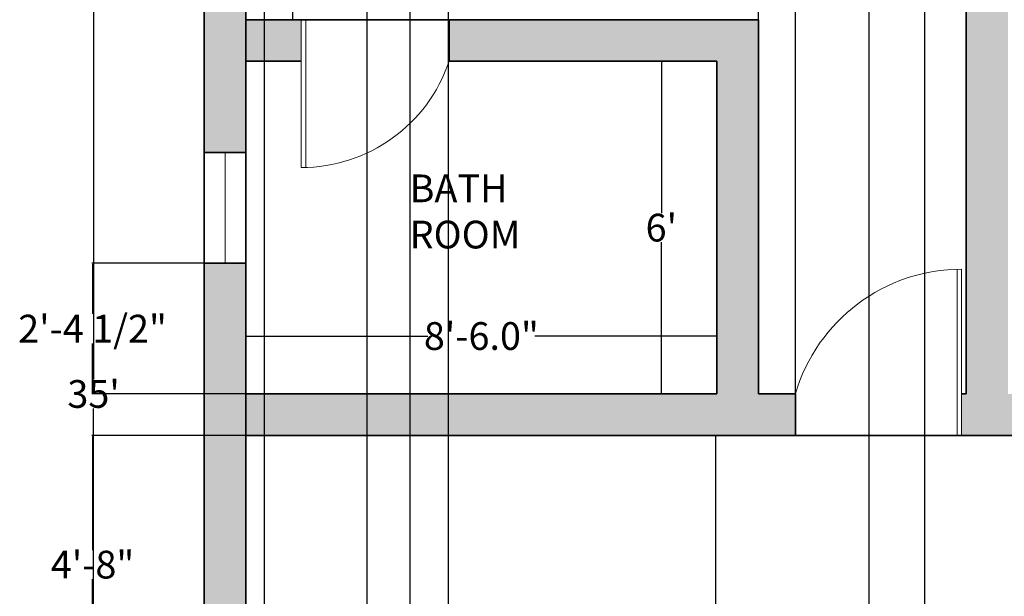
# Model space of a CAD drawing. Units: inches. Extents: x 1174 to 1615, y 3112 to 3628.
# Tile 3 of 6: x 1177 to 1390, y 3341 to 3466. Entities that reach past the tile are written whole.
import ezdxf

# ---------------------------------------------------------------- set-up
doc = ezdxf.new("R2010")
doc.units = ezdxf.units.IN
doc.header["$MEASUREMENT"] = 0
doc.layers.get('0').update_dxf_attribs({"color": 250})
for name, color, linetype, lineweight in [('A-ANNO-DIMS', 2, 'Continuous', 18), ('A-AREA-IDEN', 7, 'Continuous', 25), ('A-DOOR', 3, 'Continuous', 18), ('A-GLAZ', 4, 'Continuous', 18), ('A-WALL', 7, 'Continuous', 35)]:
    doc.layers.add(name, color=color, linetype=linetype, lineweight=lineweight)
doc.layers.add('A-WALL-PATT', color=18, linetype='Continuous', lineweight=13, true_color=0x000000)
doc.styles.get("Standard").update_dxf_attribs({"font": 'arial.ttf'})
doc.dimstyles.get("Standard").update_dxf_attribs({"dimtxt": 6, "dimasz": 0.18, "dimexe": 0.18, "dimexo": 0.0625, "dimgap": 0.09, "dimtad": 0, "dimtih": 1, "dimtoh": 1, "dimdec": 1, "dimzin": 0, "dimdsep": 46, "dimlunit": 3, "dimtxsty": 'Standard', "dimcen": 0.09, "dimadec": 0, "dimazin": 0, "dimtfac": 1, "dimtdec": 1, "dimtofl": 0, "dimtmove": 0, "dimatfit": 3, "dimfxl": 1, "dimtolj": 1, "dimtzin": 0, "dimarcsym": 0})

# ---------------------------------------------------------------- blocks, each defined once
blk = doc.blocks.new('*D4')
at = {"layer": 'A-ANNO-DIMS', "color": 0, "lineweight": -2, "transparency": 16777216}
for p, q in [((1216.6, 3595.03), (1192.51, 3595.03)), ((1192.69, 3594.85), (1192.69, 3388.18)), ((1192.69, 3175.21), (1192.69, 3381.87)), ((1216.6, 3175.03), (1192.51, 3175.03))]:
    blk.add_line(p, q, dxfattribs=at)
at = {"layer": 'A-ANNO-DIMS', "color": 0, "transparency": 16777216}
for points in [[(1192.66, 3594.85), (1192.72, 3594.85), (1192.69, 3595.03)], [(1192.66, 3175.21), (1192.72, 3175.21), (1192.69, 3175.03)]]:
    blk.add_solid(points, dxfattribs=at)
at = {"layer": 'Defpoints', "color": 0, "transparency": 16777216}
for p in [(1216.66, 3595.03), (1192.69, 3175.03), (1216.66, 3175.03)]:
    blk.add_point(p, dxfattribs=at)
at = {"layer": 'A-ANNO-DIMS', "color": 0, "transparency": 16777216, "insert": (1192.69, 3385.03), "char_height": 6, "attachment_point": 5}
blk.add_mtext("\\A1;35'", dxfattribs=at)
blk = doc.blocks.new('*D5')
at = {"layer": 'A-ANNO-DIMS', "color": 0, "lineweight": -2, "transparency": 16777216}
for p, q in [((1225.73, 3586.03), (1236.02, 3586.03)), ((1235.84, 3585.85), (1235.84, 3529.18)), ((1235.84, 3466.21), (1235.84, 3522.88)), ((1225.73, 3466.03), (1236.02, 3466.03))]:
    blk.add_line(p, q, dxfattribs=at)
at = {"layer": 'A-ANNO-DIMS', "color": 0, "transparency": 16777216}
for points in [[(1235.81, 3585.85), (1235.87, 3585.85), (1235.84, 3586.03)], [(1235.81, 3466.21), (1235.87, 3466.21), (1235.84, 3466.03)]]:
    blk.add_solid(points, dxfattribs=at)
at = {"layer": 'Defpoints', "color": 0, "transparency": 16777216}
for p in [(1225.66, 3586.03), (1225.66, 3466.03), (1235.84, 3466.03)]:
    blk.add_point(p, dxfattribs=at)
at = {"layer": 'A-ANNO-DIMS', "color": 0, "transparency": 16777216, "insert": (1235.84, 3526.03), "char_height": 6, "attachment_point": 5}
blk.add_mtext("\\A1;10'", dxfattribs=at)
blk = doc.blocks.new('*D7')
at = {"layer": 'A-ANNO-DIMS', "color": 0, "lineweight": -2, "transparency": 16777216}
for p, q in [((1225.66, 3385.09), (1225.66, 3397.75)), ((1225.84, 3397.57), (1265.1, 3397.57)), ((1327.48, 3397.57), (1288.23, 3397.57)), ((1327.66, 3385.09), (1327.66, 3397.75))]:
    blk.add_line(p, q, dxfattribs=at)
at = {"layer": 'A-ANNO-DIMS', "color": 0, "transparency": 16777216}
for points in [[(1225.84, 3397.6), (1225.84, 3397.54), (1225.66, 3397.57)], [(1327.48, 3397.6), (1327.48, 3397.54), (1327.66, 3397.57)]]:
    blk.add_solid(points, dxfattribs=at)
at = {"layer": 'Defpoints', "color": 0, "transparency": 16777216}
for p in [(1327.66, 3397.57), (1225.66, 3385.03), (1327.66, 3385.03)]:
    blk.add_point(p, dxfattribs=at)
at = {"layer": 'A-ANNO-DIMS', "color": 0, "transparency": 16777216, "insert": (1276.66, 3397.57), "char_height": 6, "attachment_point": 5}
blk.add_mtext('\\A1;8\'-6.0"', dxfattribs=at)
blk = doc.blocks.new('*D8')
at = {"layer": 'A-ANNO-DIMS', "color": 0, "lineweight": -2, "transparency": 16777216}
for p, q in [((1327.6, 3457.03), (1315.45, 3457.03)), ((1315.63, 3456.85), (1315.63, 3424.18)), ((1315.63, 3385.21), (1315.63, 3417.88)), ((1327.6, 3385.03), (1315.45, 3385.03))]:
    blk.add_line(p, q, dxfattribs=at)
at = {"layer": 'A-ANNO-DIMS', "color": 0, "transparency": 16777216}
for points in [[(1315.6, 3456.85), (1315.66, 3456.85), (1315.63, 3457.03)], [(1315.6, 3385.21), (1315.66, 3385.21), (1315.63, 3385.03)]]:
    blk.add_solid(points, dxfattribs=at)
at = {"layer": 'Defpoints', "color": 0, "transparency": 16777216}
for p in [(1327.66, 3457.03), (1315.63, 3385.03), (1327.66, 3385.03)]:
    blk.add_point(p, dxfattribs=at)
at = {"layer": 'A-ANNO-DIMS', "color": 0, "transparency": 16777216, "insert": (1315.63, 3421.03), "char_height": 6, "attachment_point": 5}
blk.add_mtext("\\A1;6'", dxfattribs=at)
blk = doc.blocks.new('*D18')
at = {"layer": 'A-ANNO-DIMS', "color": 0, "lineweight": -2, "transparency": 16777216}
for p, q in [((1225.73, 3376.03), (1327.55, 3376.03)), ((1327.37, 3375.85), (1327.37, 3283.18)), ((1327.37, 3184.21), (1327.37, 3276.88)), ((1225.73, 3184.03), (1327.55, 3184.03))]:
    blk.add_line(p, q, dxfattribs=at)
at = {"layer": 'A-ANNO-DIMS', "color": 0, "transparency": 16777216}
for points in [[(1327.34, 3375.85), (1327.4, 3375.85), (1327.37, 3376.03)], [(1327.34, 3184.21), (1327.4, 3184.21), (1327.37, 3184.03)]]:
    blk.add_solid(points, dxfattribs=at)
at = {"layer": 'Defpoints', "color": 0, "transparency": 16777216}
for p in [(1225.66, 3376.03), (1225.66, 3184.03), (1327.37, 3184.03)]:
    blk.add_point(p, dxfattribs=at)
at = {"layer": 'A-ANNO-DIMS', "color": 0, "transparency": 16777216, "insert": (1327.37, 3280.03), "char_height": 6, "attachment_point": 5}
blk.add_mtext("\\A1;16'", dxfattribs=at)
blk = doc.blocks.new('DOOR-SWING-36IN')
for p, q in [((-1, 36), (-1, 0)), ((0, 0), (0, 36)), ((0, 0), (-36, 0))]:
    blk.add_line(p, q)
blk.add_arc((0, -1.5), 37.5, 90, 163.7398)
blk = doc.blocks.new('DOOR-SWING-32IN')
for p, q in [((0, 0), (0, -32)), ((0, 0), (32, 0)), ((1, -32), (1, 0))]:
    blk.add_line(p, q)
blk.add_arc((0, 1.76), 33.76, 270, 341.4134)
blk = doc.blocks.new('VENT-WINDOW-24IN')
for p, q in [((-4.5, -24), (-4.5, 0)), ((0, 0), (0, -24)), ((4.5, 0), (4.5, -24))]:
    blk.add_line(p, q)
blk = doc.blocks.new('*D48')
at = {"layer": 'A-ANNO-DIMS', "color": 0, "lineweight": -2, "transparency": 16777216}
for p, q in [((1225.6, 3413.31), (1192.28, 3413.31)), ((1192.46, 3413.13), (1192.46, 3402.36)), ((1192.46, 3385.21), (1192.46, 3395.98)), ((1225.6, 3385.03), (1192.28, 3385.03))]:
    blk.add_line(p, q, dxfattribs=at)
at = {"layer": 'A-ANNO-DIMS', "color": 0, "transparency": 16777216}
for points in [[(1192.43, 3413.13), (1192.49, 3413.13), (1192.46, 3413.31)], [(1192.43, 3385.21), (1192.49, 3385.21), (1192.46, 3385.03)]]:
    blk.add_solid(points, dxfattribs=at)
at = {"layer": 'Defpoints', "color": 0, "transparency": 16777216}
for p in [(1192.46, 3413.31), (1225.66, 3413.31), (1225.66, 3385.03)]:
    blk.add_point(p, dxfattribs=at)
at = {"layer": 'A-ANNO-DIMS', "color": 0, "transparency": 16777216, "insert": (1192.46, 3399.17), "char_height": 6, "attachment_point": 5}
blk.add_mtext('\\A1;2\'-4 1/2"', dxfattribs=at)
blk = doc.blocks.new('*D49')
at = {"layer": 'A-ANNO-DIMS', "color": 0, "lineweight": -2, "transparency": 16777216}
for p, q in [((1225.73, 3376.03), (1589.04, 3376.03)), ((1588.86, 3375.85), (1588.86, 3351.02)), ((1588.86, 3319.81), (1588.86, 3344.64)), ((1225.73, 3319.63), (1589.04, 3319.63))]:
    blk.add_line(p, q, dxfattribs=at)
at = {"layer": 'A-ANNO-DIMS', "color": 0, "transparency": 16777216}
for points in [[(1588.83, 3375.85), (1588.89, 3375.85), (1588.86, 3376.03)], [(1588.83, 3319.81), (1588.89, 3319.81), (1588.86, 3319.63)]]:
    blk.add_solid(points, dxfattribs=at)
at = {"layer": 'Defpoints', "color": 0, "transparency": 16777216}
for p in [(1225.66, 3376.03), (1225.66, 3319.63), (1588.86, 3319.63)]:
    blk.add_point(p, dxfattribs=at)
at = {"layer": 'A-ANNO-DIMS', "color": 0, "transparency": 16777216, "insert": (1588.86, 3347.83), "char_height": 6, "attachment_point": 5}
blk.add_mtext('\\A1;4\'-8 1/2"', dxfattribs=at)
blk = doc.blocks.new('*D52')
at = {"layer": 'A-ANNO-DIMS', "color": 0, "lineweight": -2, "transparency": 16777216}
for p, q in [((1555.6, 3376.03), (1192.28, 3376.03)), ((1192.46, 3375.85), (1192.46, 3351.26)), ((1192.46, 3320.35), (1192.46, 3344.95)), ((1555.6, 3320.17), (1192.28, 3320.17))]:
    blk.add_line(p, q, dxfattribs=at)
at = {"layer": 'A-ANNO-DIMS', "color": 0, "transparency": 16777216}
for points in [[(1192.43, 3375.85), (1192.49, 3375.85), (1192.46, 3376.03)], [(1192.43, 3320.35), (1192.49, 3320.35), (1192.46, 3320.17)]]:
    blk.add_solid(points, dxfattribs=at)
at = {"layer": 'Defpoints', "color": 0, "transparency": 16777216}
for p in [(1555.66, 3376.03), (1192.46, 3320.17), (1555.66, 3320.17)]:
    blk.add_point(p, dxfattribs=at)
at = {"layer": 'A-ANNO-DIMS', "color": 0, "transparency": 16777216, "insert": (1192.46, 3348.1), "char_height": 6, "attachment_point": 5}
blk.add_mtext('\\A1;4\'-8"', dxfattribs=at)
blk = doc.blocks.new('*D56')
at = {"layer": 'A-ANNO-DIMS', "color": 0, "lineweight": -2, "transparency": 16777216}
for p, q in [((1336.66, 3385.09), (1336.66, 3619.41)), ((1336.84, 3619.23), (1344.48, 3619.23)), ((1344.66, 3385.09), (1344.66, 3619.41)), ((1344.66, 3619.23), (1344.84, 3619.23))]:
    blk.add_line(p, q, dxfattribs=at)
at = {"layer": 'A-ANNO-DIMS', "color": 0, "transparency": 16777216}
for points in [[(1336.84, 3619.26), (1336.84, 3619.2), (1336.66, 3619.23)], [(1344.48, 3619.26), (1344.48, 3619.2), (1344.66, 3619.23)]]:
    blk.add_solid(points, dxfattribs=at)
at = {"layer": 'Defpoints', "color": 0, "transparency": 16777216}
for p in [(1344.66, 3619.23), (1336.66, 3385.03), (1344.66, 3385.03)]:
    blk.add_point(p, dxfattribs=at)
at = {"layer": 'A-ANNO-DIMS', "color": 0, "transparency": 16777216, "insert": (1352.91, 3619.23), "char_height": 6, "attachment_point": 5}
blk.add_mtext('\\A1;0\'-8"', dxfattribs=at)
blk = doc.blocks.new('*D58')
at = {"layer": 'A-ANNO-DIMS', "color": 0, "lineweight": -2, "transparency": 16777216}
for p, q in [((1360.66, 3184.09), (1360.66, 3619.41)), ((1360.84, 3619.23), (1372.48, 3619.23)), ((1372.66, 3184.09), (1372.66, 3619.41)), ((1372.66, 3619.23), (1372.84, 3619.23))]:
    blk.add_line(p, q, dxfattribs=at)
at = {"layer": 'A-ANNO-DIMS', "color": 0, "transparency": 16777216}
for points in [[(1360.84, 3619.26), (1360.84, 3619.2), (1360.66, 3619.23)], [(1372.48, 3619.26), (1372.48, 3619.2), (1372.66, 3619.23)]]:
    blk.add_solid(points, dxfattribs=at)
at = {"layer": 'Defpoints', "color": 0, "transparency": 16777216}
for p in [(1372.66, 3619.23), (1360.66, 3184.03), (1372.66, 3184.03)]:
    blk.add_point(p, dxfattribs=at)
at = {"layer": 'A-ANNO-DIMS', "color": 0, "transparency": 16777216, "insert": (1380.63, 3619.23), "char_height": 6, "attachment_point": 5}
blk.add_mtext('\\A1;1\'-0"', dxfattribs=at)
blk = doc.blocks.new('*D60')
at = {"layer": 'A-ANNO-DIMS', "color": 0, "lineweight": -2, "transparency": 16777216}
for p, q in [((1229.72, 3290.15), (1229.72, 3619.41)), ((1229.9, 3619.23), (1230.72, 3619.23)), ((1251.77, 3619.23), (1250.95, 3619.23)), ((1251.95, 3292.11), (1251.95, 3619.41))]:
    blk.add_line(p, q, dxfattribs=at)
at = {"layer": 'A-ANNO-DIMS', "color": 0, "transparency": 16777216}
for points in [[(1229.9, 3619.26), (1229.9, 3619.2), (1229.72, 3619.23)], [(1251.77, 3619.26), (1251.77, 3619.2), (1251.95, 3619.23)]]:
    blk.add_solid(points, dxfattribs=at)
at = {"layer": 'Defpoints', "color": 0, "transparency": 16777216}
for p in [(1251.95, 3619.23), (1251.95, 3292.05), (1229.72, 3290.09)]:
    blk.add_point(p, dxfattribs=at)
at = {"layer": 'A-ANNO-DIMS', "color": 0, "transparency": 16777216, "insert": (1240.84, 3619.23), "char_height": 6, "attachment_point": 5}
blk.add_mtext('\\A1;1\'-10"', dxfattribs=at)
blk = doc.blocks.new('*D64')
at = {"layer": 'A-ANNO-DIMS', "color": 0, "lineweight": -2, "transparency": 16777216}
for p, q in [((1251.95, 3292.11), (1251.95, 3619.41)), ((1252.13, 3619.23), (1269.39, 3619.23)), ((1269.57, 3281.81), (1269.57, 3619.41)), ((1269.57, 3619.23), (1269.75, 3619.23))]:
    blk.add_line(p, q, dxfattribs=at)
at = {"layer": 'A-ANNO-DIMS', "color": 0, "transparency": 16777216}
for points in [[(1252.13, 3619.26), (1252.13, 3619.2), (1251.95, 3619.23)], [(1269.39, 3619.26), (1269.39, 3619.2), (1269.57, 3619.23)]]:
    blk.add_solid(points, dxfattribs=at)
at = {"layer": 'Defpoints', "color": 0, "transparency": 16777216}
for p in [(1269.57, 3619.23), (1251.95, 3292.05), (1269.57, 3281.75)]:
    blk.add_point(p, dxfattribs=at)
at = {"layer": 'A-ANNO-DIMS', "color": 0, "transparency": 16777216, "insert": (1284.52, 3619.23), "char_height": 6, "attachment_point": 5}
blk.add_mtext('\\A1;1\'-5 1/2"', dxfattribs=at)
blk = doc.blocks.new('*D69')
at = {"layer": 'A-ANNO-DIMS', "color": 0, "lineweight": -2, "transparency": 16777216}
for p, q in [((1225.66, 3585.97), (1225.66, 3120.65)), ((1261.16, 3585.86), (1261.16, 3120.65)), ((1225.84, 3120.83), (1225.98, 3120.83)), ((1260.98, 3120.83), (1260.85, 3120.83))]:
    blk.add_line(p, q, dxfattribs=at)
at = {"layer": 'A-ANNO-DIMS', "color": 0, "transparency": 16777216}
for points in [[(1225.84, 3120.86), (1225.84, 3120.8), (1225.66, 3120.83)], [(1260.98, 3120.86), (1260.98, 3120.8), (1261.16, 3120.83)]]:
    blk.add_solid(points, dxfattribs=at)
at = {"layer": 'Defpoints', "color": 0, "transparency": 16777216}
for p in [(1225.66, 3586.03), (1261.16, 3585.93), (1261.16, 3120.83)]:
    blk.add_point(p, dxfattribs=at)
at = {"layer": 'A-ANNO-DIMS', "color": 0, "transparency": 16777216, "insert": (1243.41, 3120.83), "char_height": 6, "attachment_point": 5}
blk.add_mtext('\\A1;2\'-11 1/2"', dxfattribs=at)
blk = doc.blocks.new('*D71')
at = {"layer": 'A-ANNO-DIMS', "color": 0, "lineweight": -2, "transparency": 16777216}
for p, q in [((1225.66, 3283.7), (1225.66, 3619.41)), ((1225.84, 3619.23), (1229.54, 3619.23)), ((1229.72, 3290.15), (1229.72, 3619.41)), ((1229.72, 3619.23), (1229.9, 3619.23))]:
    blk.add_line(p, q, dxfattribs=at)
at = {"layer": 'A-ANNO-DIMS', "color": 0, "transparency": 16777216}
for points in [[(1225.84, 3619.26), (1225.84, 3619.2), (1225.66, 3619.23)], [(1229.54, 3619.26), (1229.54, 3619.2), (1229.72, 3619.23)]]:
    blk.add_solid(points, dxfattribs=at)
at = {"layer": 'Defpoints', "color": 0, "transparency": 16777216}
for p in [(1229.72, 3619.23), (1229.72, 3290.09), (1225.66, 3283.63)]:
    blk.add_point(p, dxfattribs=at)
at = {"layer": 'A-ANNO-DIMS', "color": 0, "transparency": 16777216, "insert": (1237.97, 3619.23), "char_height": 6, "attachment_point": 5}
blk.add_mtext('\\A1;0\'-4"', dxfattribs=at)

msp = doc.modelspace()

# ---------------------------------------------------------------- hatches: boundary and pattern name
at = {"layer": 'A-WALL-PATT'}
h = msp.add_hatch(color=256, dxfattribs=at)
h.dxf.hatch_style = 1
h.paths.add_polyline_path([(1564.66, 3595.03), (1216.66, 3595.03), (1216.66, 3564.55), (1225.66, 3564.55), (1225.66, 3586.03), (1381.66, 3586.03), (1381.66, 3385.03), (1380.66, 3385.03), (1380.66, 3376.03), (1381.66, 3376.03), (1407.66, 3376.03), (1407.66, 3385.03), (1390.66, 3385.03), (1390.66, 3586.03), (1555.66, 3586.03), (1555.66, 3558.83), (1564.66, 3558.83)])
h.paths.add_polyline_path([(1564.66, 3408.64), (1555.66, 3408.64), (1555.66, 3385.03), (1453.66, 3385.03), (1453.66, 3457.03), (1465.66, 3457.03), (1465.66, 3466.03), (1453.66, 3466.03), (1444.66, 3466.03), (1444.66, 3385.03), (1443.66, 3385.03), (1443.66, 3376.03), (1444.66, 3376.03), (1555.66, 3376.03), (1555.66, 3320.17), (1564.66, 3320.17)])
h.paths.add_polyline_path([(1564.66, 3522.83), (1555.66, 3522.83), (1555.66, 3466.03), (1497.66, 3466.03), (1497.66, 3457.03), (1555.66, 3457.03), (1555.66, 3432.64), (1564.66, 3432.64)], flags=17)
h.paths.add_polyline_path([(1344.66, 3385.03), (1336.66, 3385.03), (1336.66, 3466.03), (1269.66, 3466.03), (1269.66, 3457.03), (1327.66, 3457.03), (1327.66, 3385.03), (1225.66, 3385.03), (1225.66, 3413.31), (1216.66, 3413.31), (1216.66, 3319.63), (1225.66, 3319.63), (1225.66, 3376.03), (1344.66, 3376.03)])
h.paths.add_polyline_path([(1237.66, 3466.03), (1225.66, 3466.03), (1225.66, 3528.55), (1216.66, 3528.55), (1216.66, 3437.31), (1225.66, 3437.31), (1225.66, 3457.03), (1237.66, 3457.03)], flags=17)
h.paths.add_polyline_path([(1265.25, 3184.03), (1225.66, 3184.03), (1225.66, 3283.63), (1216.66, 3283.63), (1216.66, 3175.03), (1265.25, 3175.03)])
h.paths.add_polyline_path([(1372.66, 3184.03), (1360.66, 3184.03), (1360.66, 3268.03), (1376.66, 3268.03), (1376.66, 3277.03), (1360.66, 3277.03), (1360.66, 3313.03), (1351.66, 3313.03), (1351.66, 3184.03), (1301.25, 3184.03), (1301.25, 3175.03), (1372.66, 3175.03)])
h.paths.add_polyline_path([(1460.02, 3184.03), (1429.66, 3184.03), (1429.66, 3277.03), (1408.66, 3277.03), (1408.66, 3268.03), (1420.66, 3268.03), (1420.66, 3184.03), (1408.66, 3184.03), (1408.66, 3175.03), (1460.02, 3175.03)])
h.paths.add_polyline_path([(1564.66, 3284.17), (1555.66, 3284.17), (1555.66, 3184.03), (1520.02, 3184.03), (1520.02, 3175.03), (1564.66, 3175.03)])

# ---------------------------------------------------------------- linework, layer by layer
at = {"layer": 'A-DOOR'}
for p, q in [((1237.66, 3434.03), (1237.66, 3466.03)), ((1380.66, 3412.03), (1380.66, 3376.03))]:
    msp.add_line(p, q, dxfattribs=at)
at = {"layer": 'A-WALL'}
for p, q in [((1216.66, 3595.03), (1216.66, 3175.03)), ((1225.66, 3586.03), (1225.66, 3466.03)), ((1381.66, 3586.03), (1381.66, 3385.03)), ((1225.66, 3466.03), (1336.66, 3466.03)), ((1225.66, 3466.03), (1237.66, 3466.03)), ((1269.66, 3466.03), (1269.66, 3457.03)), ((1336.66, 3466.03), (1336.66, 3385.03)), ((1225.66, 3457.03), (1237.66, 3457.03)), ((1225.66, 3457.03), (1225.66, 3385.03)), ((1269.66, 3457.03), (1327.66, 3457.03)), ((1327.66, 3457.03), (1327.66, 3385.03)), ((1216.66, 3437.31), (1225.66, 3437.31)), ((1225.66, 3413.31), (1216.66, 3413.31)), ((1225.66, 3385.03), (1327.66, 3385.03)), ((1336.66, 3385.03), (1344.66, 3385.03)), ((1344.66, 3376.03), (1344.66, 3385.03)), ((1380.66, 3385.03), (1381.66, 3385.03)), ((1225.66, 3376.03), (1555.66, 3376.03)), ((1225.66, 3376.03), (1225.66, 3184.03)), ((1381.66, 3376.03), (1380.66, 3376.03))]:
    msp.add_line(p, q, dxfattribs=at)

# ---------------------------------------------------------------- block references
at = {"layer": 'A-DOOR'}
for name, p in [('DOOR-SWING-32IN', (1237.66, 3466.03)), ('DOOR-SWING-36IN', (1380.66, 3376.03))]:
    msp.add_blockref(name, p, dxfattribs=at)
at = {"layer": 'A-GLAZ'}
msp.add_blockref('VENT-WINDOW-24IN', (1221.16, 3437.31), dxfattribs=at)

# ---------------------------------------------------------------- texts
at = {"layer": 'A-AREA-IDEN', "insert": (1261.12, 3432.53), "char_height": 6, "attachment_point": 1}
msp.add_mtext_dynamic_manual_height_columns('BATH \\PROOM', width=55.5508, gutter_width=1, heights=[0], dxfattribs=at)

# ---------------------------------------------------------------- dimensions: what is measured, and where the dimension line sits
at = {"layer": 'A-ANNO-DIMS'}
for base, p1, p2, override, picture, middle in [((1269.57, 3619.23), (1251.95, 3292.05), (1269.57, 3281.75), {"dimdec": 1, "dimlfac": 1, "dimrnd": 0, "dimzin": 1, "dimdsep": 46, "dimlunit": 4, "dimfrac": 2}, '*D64', (1284.52, 3619.23)), ((1229.72, 3619.23), (1225.66, 3283.63), (1229.72, 3290.09), {"dimdec": 1, "dimlfac": 1, "dimrnd": 0, "dimzin": 1, "dimdsep": 46, "dimlunit": 4, "dimfrac": 2}, '*D71', (1237.97, 3619.23)), ((1251.95, 3619.23), (1229.72, 3290.09), (1251.95, 3292.05), {"dimdec": 1, "dimlfac": 1, "dimrnd": 0, "dimzin": 1, "dimdsep": 46, "dimlunit": 4, "dimfrac": 2}, '*D60', (1240.84, 3619.23)), ((1344.66, 3619.23), (1336.66, 3385.03), (1344.66, 3385.03), {"dimdec": 1, "dimlfac": 1, "dimrnd": 0, "dimzin": 1, "dimdsep": 46, "dimlunit": 4, "dimfrac": 2}, '*D56', (1352.91, 3619.23)), ((1372.66, 3619.23), (1360.66, 3184.03), (1372.66, 3184.03), {"dimdec": 1, "dimlfac": 1, "dimrnd": 0, "dimzin": 1, "dimdsep": 46, "dimlunit": 4, "dimfrac": 2}, '*D58', (1380.63, 3619.23)), ((1261.16, 3120.83), (1225.66, 3586.03), (1261.16, 3585.93), {"dimdec": 1, "dimlfac": 1, "dimrnd": 0, "dimzin": 1, "dimdsep": 46, "dimlunit": 4, "dimfrac": 2}, '*D69', (1243.41, 3120.83)), ((1327.66, 3397.57), (1225.66, 3385.03), (1327.66, 3385.03), {"dimclrd": 0, "dimclre": 0, "dimclrt": 0}, '*D7', (1276.66, 3397.57))]:
    dim = msp.add_linear_dim(base=base, p1=p1, p2=p2, dimstyle='Standard', override=override, dxfattribs=at)
    dim.commit()
    dim.dimension.update_dxf_attribs({"geometry": picture, "text_midpoint": middle})
for base, p1, p2, override, picture, middle in [((1192.69, 3175.03), (1216.66, 3595.03), (1216.66, 3175.03), {"dimclrd": 0, "dimclre": 0, "dimclrt": 0}, '*D4', (1192.69, 3385.03)), ((1235.84, 3466.03), (1225.66, 3586.03), (1225.66, 3466.03), {"dimclrd": 0, "dimclre": 0, "dimclrt": 0}, '*D5', (1235.84, 3526.03)), ((1315.63, 3385.03), (1327.66, 3457.03), (1327.66, 3385.03), {"dimclrd": 0, "dimclre": 0, "dimclrt": 0}, '*D8', (1315.63, 3421.03)), ((1192.46, 3413.31), (1225.66, 3385.03), (1225.66, 3413.31), {"dimdec": 1, "dimlfac": 1, "dimrnd": 0, "dimzin": 1, "dimdsep": 46, "dimlunit": 4, "dimfrac": 2}, '*D48', (1192.46, 3399.17)), ((1192.46, 3320.17), (1555.66, 3376.03), (1555.66, 3320.17), {"dimdec": 1, "dimlfac": 1, "dimrnd": 0, "dimzin": 1, "dimdsep": 46, "dimlunit": 4, "dimfrac": 2}, '*D52', (1192.46, 3348.1)), ((1327.37, 3184.03), (1225.66, 3376.03), (1225.66, 3184.03), {"dimclrd": 0, "dimclre": 0, "dimclrt": 0}, '*D18', (1327.37, 3280.03)), ((1588.86, 3319.63), (1225.66, 3376.03), (1225.66, 3319.63), {"dimdec": 1, "dimlfac": 1, "dimrnd": 0, "dimzin": 1, "dimdsep": 46, "dimlunit": 4, "dimfrac": 2}, '*D49', (1588.86, 3347.83))]:
    dim = msp.add_linear_dim(base=base, p1=p1, p2=p2, angle=90, dimstyle='Standard', override=override, dxfattribs=at)
    dim.commit()
    dim.dimension.update_dxf_attribs({"geometry": picture, "text_midpoint": middle})

doc.saveas('drawing.dxf')
